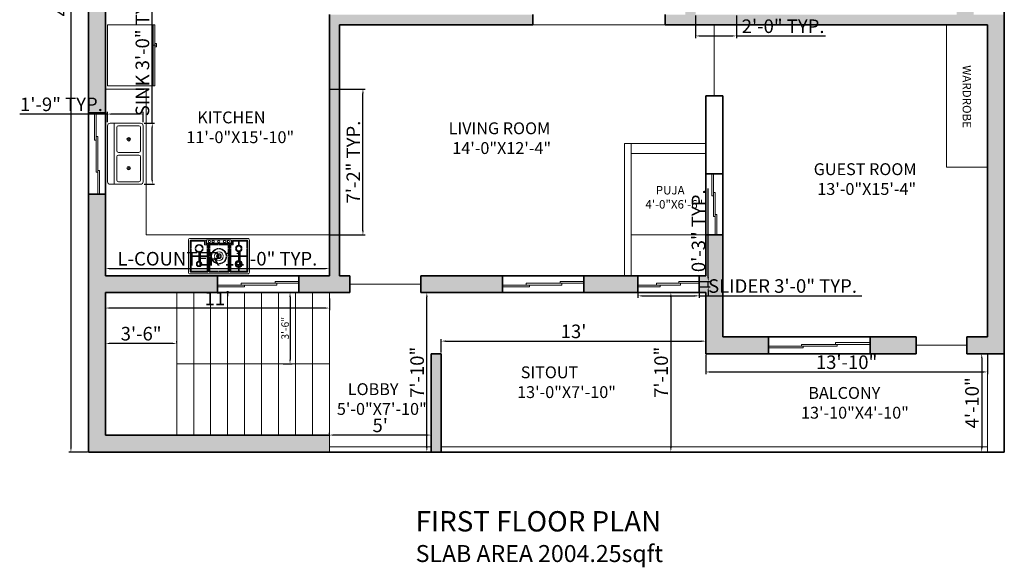
# Model space of a CAD drawing. Units: inches. Extents: x 3491 to 6898, y 1360 to 2019.
# Tile 4 of 9: x 4120 to 4700, y 1360 to 1683. Entities that reach past the tile are written whole.
import ezdxf

# ---------------------------------------------------------------- set-up
doc = ezdxf.new("R2010")
doc.units = ezdxf.units.IN
for name, color, linetype, lineweight in [('A-ANNO-DIMS', 2, 'Continuous', 18), ('A-ANNO-TEXT', 7, 'Continuous', 18), ('A-ANNO-TITL', 7, 'Continuous', 30), ('A-AREA-IDEN', 7, 'Continuous', 18), ('A-DOOR', 4, 'Continuous', 18), ('A-EQPM', 8, 'Continuous', 18), ('A-FLOR-CASE', 8, 'Continuous', 18), ('A-FLOR-FIXT', 8, 'Continuous', 18), ('A-FLOR-RAL', 7, 'Continuous', 18), ('A-FLOR-STRS', 7, 'Continuous', 18), ('A-GLAZ', 5, 'Continuous', 18), ('A-WALL', 7, 'Continuous', 35), ('A-WALL-PATT', 8, 'Continuous', 13)]:
    doc.layers.add(name, color=color, linetype=linetype, lineweight=lineweight)
doc.layers.add('A-WALL-OPEN', color=251, linetype='Continuous', lineweight=13, true_color=0x636466)
doc.styles.get("Standard").update_dxf_attribs({"font": 'arial.ttf'})
doc.dimstyles.new('ISO-25', dxfattribs={"dimtxt": 8, "dimasz": 2.5, "dimexe": 1.25, "dimexo": 0.625, "dimtad": 1, "dimdec": 1, "dimlunit": 3, "dimtxsty": 'Standard', "dimcen": 2.5, "dimclrt": 1, "dimadec": 0, "dimazin": 0, "dimtfac": 1, "dimtdec": 1, "dimtmove": 0, "dimatfit": 3, "dimfxl": 1, "dimarcsym": 0})

# ---------------------------------------------------------------- blocks, each defined once
blk = doc.blocks.new('*D17')
at = {"layer": 'A-ANNO-DIMS', "color": 0, "lineweight": -2, "transparency": 16777216}
for p, q in [((4159.68, 1972.37), (4148.67, 1972.37)), ((4149.92, 1969.87), (4149.92, 1430.87)), ((4159.68, 1428.37), (4148.67, 1428.37))]:
    blk.add_line(p, q, dxfattribs=at)
at = {"layer": 'A-ANNO-DIMS', "color": 0, "transparency": 16777216}
for points in [[(4149.51, 1969.87), (4150.34, 1969.87), (4149.92, 1972.37)], [(4149.51, 1430.87), (4150.34, 1430.87), (4149.92, 1428.37)]]:
    blk.add_solid(points, dxfattribs=at)
at = {"layer": 'Defpoints', "color": 0, "transparency": 16777216}
for p in [(4160.3, 1972.37), (4149.92, 1428.37), (4160.3, 1428.37)]:
    blk.add_point(p, dxfattribs=at)
at = {"layer": 'A-ANNO-DIMS', "color": 0, "transparency": 16777216, "insert": (4145.23, 1700.37), "char_height": 8, "attachment_point": 5, "rotation": 90}
blk.add_mtext('45\'-4"', dxfattribs=at)
blk = doc.blocks.new('*D14')
at = {"layer": 'A-ANNO-DIMS', "color": 0, "lineweight": -2, "transparency": 16777216}
for p, q in [((4170.3, 1493.03), (4170.3, 1493.65)), ((4209.8, 1492.4), (4172.8, 1492.4)), ((4212.3, 1493.03), (4212.3, 1493.65))]:
    blk.add_line(p, q, dxfattribs=at)
at = {"layer": 'A-ANNO-DIMS', "color": 0, "transparency": 16777216}
for points in [[(4172.8, 1492.82), (4172.8, 1491.99), (4170.3, 1492.4)], [(4209.8, 1492.82), (4209.8, 1491.99), (4212.3, 1492.4)]]:
    blk.add_solid(points, dxfattribs=at)
at = {"layer": 'Defpoints', "color": 0, "transparency": 16777216}
for p in [(4170.3, 1492.4), (4170.3, 1492.4), (4212.3, 1492.4)]:
    blk.add_point(p, dxfattribs=at)
at = {"layer": 'A-ANNO-DIMS', "color": 0, "transparency": 16777216, "insert": (4191.3, 1497.12), "char_height": 8, "attachment_point": 5}
blk.add_mtext('3\'-6"', dxfattribs=at)
blk = doc.blocks.new('*D12')
at = {"layer": 'A-ANNO-DIMS', "color": 0, "lineweight": -2, "transparency": 16777216}
for p, q in [((4275.02, 1522.37), (4280.36, 1522.37)), ((4279.11, 1519.87), (4279.11, 1482.87)), ((4275.02, 1480.37), (4280.36, 1480.37))]:
    blk.add_line(p, q, dxfattribs=at)
at = {"layer": 'A-ANNO-DIMS', "color": 0, "transparency": 16777216}
for points in [[(4278.69, 1519.87), (4279.53, 1519.87), (4279.11, 1522.37)], [(4278.69, 1482.87), (4279.53, 1482.87), (4279.11, 1480.37)]]:
    blk.add_solid(points, dxfattribs=at)
at = {"layer": 'Defpoints', "color": 0, "transparency": 16777216}
for p in [(4274.39, 1522.37), (4274.39, 1480.37), (4279.11, 1480.37)]:
    blk.add_point(p, dxfattribs=at)
at = {"layer": 'A-ANNO-DIMS', "color": 0, "transparency": 16777216, "insert": (4276.22, 1501.37), "char_height": 8, "attachment_point": 5, "rotation": 90}
blk.add_mtext('{\\H0.55556x;3\'-6"}', dxfattribs=at)
blk = doc.blocks.new('STOVE')
for p, q in [((11.85, 19.7), (11.55, 19.7)), ((11.55, 16.92), (11.55, 19.7)), ((11.85, 16.92), (11.85, 19.7)), ((-11.85, 13.73), (-11.85, 7.62)), ((-11.85, 13.73), (-11.55, 13.73)), ((-11.55, 13.73), (-11.55, 7.62)), ((11.85, 16.92), (11.55, 16.92)), ((11.85, 13.23), (11.55, 13.23)), ((11.55, 13.23), (11.55, 7.57)), ((11.85, 13.23), (11.85, 7.57)), ((-11.85, 10.75), (-16.4, 10.75)), ((-11.85, 10.25), (-16.4, 10.25)), ((-11.85, 7.62), (-11.55, 7.62)), ((-7, 10.75), (-11.55, 10.75)), ((-7, 10.25), (-11.55, 10.25)), ((7, 10.75), (11.55, 10.75)), ((7, 10.25), (11.55, 10.25)), ((11.85, 7.57), (11.55, 7.57)), ((11.85, 10.75), (16.4, 10.75)), ((11.85, 10.25), (16.4, 10.25)), ((-7, 3.9), (-8.4, 3.9)), ((-7.8, 3.3), (-7.8, 1)), ((-6.4, 3.3), (-7.8, 3.3)), ((7.3, 2.8), (-7.3, 2.8)), ((-7.3, 2.8), (-7.3, 0.8)), ((7.3, 0.8), (-7.3, 0.8)), ((-5.4, 3.9), (-6, 3.9)), ((-5.4, 3.9), (-0.15, 3.9)), ((0.15, 3.9), (5.4, 3.9)), ((6.4, 3.3), (7.8, 3.3)), ((7, 3.9), (8.4, 3.9)), ((7.3, 2.8), (7.3, 0.8)), ((7.8, 3.3), (7.8, 1)), ((8.4, 3.9), (8.4, 1.6)), ((11.85, 4.28), (11.55, 4.28)), ((11.55, 4.28), (11.55, 1.3)), ((11.85, 1.3), (11.55, 1.3)), ((11.85, 4.28), (11.85, 1.3))]:
    blk.add_line(p, q)
for points in [[(-17, 21), (17, 21, -0.414214), (18, 20), (18, 1, -0.414214), (17, 0), (-17, 0, -0.414214), (-18, 1), (-18, 20, -0.414214)], [(6, 3.3), (-6, 3.3), (-6, 19.4, -0.414214), (-5.4, 20), (5.4, 20, -0.414214), (6, 19.4)]]:
    blk.add_lwpolyline(points, format="xyb", close=True)
for points in [[(-7.8, 1), (-16.4, 1, -0.414214), (-17, 1.6), (-17, 19.4, -0.414214), (-16.4, 20), (-7, 20, -0.414214), (-6.4, 19.4), (-6.4, 3.3)], [(6.4, 19.4, -0.414214), (7, 20), (16.4, 20, -0.414214), (17, 19.4), (17, 1.6, -0.414214), (16.4, 1), (7.8, 1)]]:
    blk.add_lwpolyline(points, format="xyb")
for points in [[(-16.4, 15.22), (-16.4, 19.4), (-11.85, 19.4)], [(-11.55, 19.4), (-7, 19.4), (-7, 15.22)], [(-5.4, 15.22), (-5.4, 19.4), (-0.15, 19.4)], [(0.15, 19.4), (5.4, 19.4), (5.4, 15.22)], [(6.4, 3.3), (6.4, 19.4)], [(7, 15.22), (7, 19.4), (11.55, 19.4)], [(11.85, 19.4), (16.4, 19.4), (16.4, 15.22)], [(-16.4, 6.08), (-16.4, 14.92)], [(-7, 14.92), (-7, 6.08)], [(-5.4, 10.65), (-5.4, 14.92)], [(5.4, 14.92), (5.4, 10.65)], [(7, 6.08), (7, 14.92)], [(16.4, 14.92), (16.4, 6.08)], [(-5.4, 6.08), (-5.4, 10.35)], [(5.4, 10.35), (5.4, 6.08)], [(-11.85, 1.6), (-16.4, 1.6), (-16.4, 5.77)], [(-8.4, 3.9), (-8.4, 1.6), (-11.55, 1.6)], [(-7, 5.77), (-7, 3.9)], [(-5.4, 3.9), (-5.4, 5.77)], [(5.4, 5.77), (5.4, 3.9)], [(7, 3.9), (7, 5.77)], [(11.55, 1.6), (8.4, 1.6)], [(16.4, 5.77), (16.4, 1.6), (11.85, 1.6)]]:
    blk.add_lwpolyline(points)
for centre, radius in [((-11.7, 15.07), 1.1), ((0, 10.5), 1.4), ((11.7, 15.07), 1.6), ((11.7, 15.07), 1.1), ((0, 10.5), 0.8), ((11.7, 5.93), 1.4), ((-5.49, 1.8), 0.6), ((-3.3, 1.8), 0.6), ((0, 1.8), 0.6), ((3.39, 1.8), 0.6), ((5.57, 1.8), 0.6)]:
    blk.add_circle(centre, radius)
for centre, radius, start, end in [((-11.7, 15.07), 1.6, 95.37938, 174.62062), ((-11.7, 15.07), 1.6, 185.37938, 264.62062), ((-11.7, 15.07), 1.6, 5.37938, 84.62062), ((-11.7, 15.07), 1.6, 275.37938, 354.62062), ((0, 10.5), 4.6, 91.86867, 178.13133), ((0, 10.5), 4.3, 91.9991, 178.0009), ((0, 10.5), 2.6, 93.30736, 176.69264), ((0, 10.5), 4.6, 1.86867, 88.13133), ((0, 10.5), 4.3, 1.9991, 88.0009), ((0, 10.5), 2.6, 3.30736, 86.69264), ((11.7, 15.07), 2.1, 94.09604, 175.90396), ((11.7, 15.07), 2.1, 184.09604, 265.90396), ((11.7, 15.07), 2.1, 4.09604, 85.90396), ((11.7, 15.07), 2.1, 274.09604, 355.90396), ((-11.7, 5.93), 2.4, 93.58332, 176.41668), ((-11.7, 5.93), 2, 94.30122, 175.69878), ((-11.7, 5.93), 2.4, 3.58332, 86.41668), ((-11.7, 5.93), 2, 4.30122, 85.69878), ((0, 10.5), 4.6, 181.86867, 268.13133), ((0, 10.5), 4.3, 181.9991, 268.0009), ((0, 10.5), 2.6, 183.30736, 266.69264), ((0, 10.5), 4.6, 271.86867, 358.13133), ((0, 10.5), 4.3, 271.9991, 358.0009), ((0, 10.5), 2.6, 273.30736, 356.69264), ((11.7, 5.93), 1.9, 94.52806, 175.47194), ((11.7, 5.93), 1.9, 4.52806, 85.47194), ((-11.7, 5.93), 2.4, 183.58332, 266.41668), ((-11.7, 5.93), 2, 184.30122, 265.69878), ((-11.7, 5.93), 2.4, 273.58332, 356.41668), ((-11.7, 5.93), 2, 274.30122, 355.69878), ((-5.49, 1.8), 0.846, 89.99794, 270), ((-3.3, 1.8), 0.846, 89.99794, 270), ((0, 1.8), 0.846, 89.99794, 270), ((3.39, 1.8), 0.846, 89.99794, 270), ((5.57, 1.8), 0.846, 89.99794, 270), ((11.7, 5.93), 1.9, 184.52806, 265.47194), ((11.7, 5.93), 1.9, 274.52806, 355.47194)]:
    blk.add_arc(centre, radius, start, end)
blk = doc.blocks.new('Sink-double - 36 in top')
for p, q in [((-18, -4), (18, -4)), ((-0.75, -18.5), (-0.75, -6.5)), ((0.75, -6.5), (0.75, -18.5))]:
    blk.add_line(p, q)
for points in [[(-16.5, 0), (16.5, 0)], [(-18, -19.5), (-18, -1.5)], [(-15.5, -5.5), (-1.75, -5.5)], [(1.75, -5.5), (15.5, -5.5)], [(18, -1.5), (18, -19.5)], [(-16.5, -18.5), (-16.5, -6.5)], [(16.5, -6.5), (16.5, -18.5)], [(16.5, -21), (-16.5, -21)], [(-1.75, -19.5), (-15.5, -19.5)], [(15.5, -19.5), (1.75, -19.5)]]:
    blk.add_lwpolyline(points)
for centre, radius in [((-8.5, -12.5), 1), ((8.5, -12.5), 1), ((-8.5, -12.5), 0.5), ((8.5, -12.5), 0.5)]:
    blk.add_circle(centre, radius)
for centre, radius, start, end in [((-16.5, -1.5), 1.5, 90, 180), ((16.5, -1.5), 1.5, 0, 90), ((-15.5, -6.5), 1, 90, 180), ((-1.75, -6.5), 1, 0, 90), ((1.75, -6.5), 1, 90, 180), ((15.5, -6.5), 1, 0, 90), ((-16.5, -19.5), 1.5, 180, 270), ((-15.5, -18.5), 1, 180, 270), ((-1.75, -18.5), 1, 270, 0), ((1.75, -18.5), 1, 180, 270), ((15.5, -18.5), 1, 270, 0), ((16.5, -19.5), 1.5, 270, 0)]:
    blk.add_arc(centre, radius, start, end)
blk = doc.blocks.new('Refrigerator-2 door - 36 in top')
for p, q in [((0, -26.999999), (36, -26.999999)), ((11, -27.999999), (11, -28.999999)), ((11, -28.999999), (13, -28.999999)), ((12, -26.999999), (12, -28.999999)), ((13, -28.999999), (13, -27.999999))]:
    blk.add_line(p, q)
blk.add_lwpolyline([(0, -27.999999), (0, 0), (36, 0), (36, -27.999999)], close=True)
blk = doc.blocks.new('*D18')
at = {"layer": 'A-ANNO-DIMS', "color": 0, "lineweight": -2, "transparency": 16777216}
for p, q in [((4170.3, 1521.74), (4170.3, 1512.03)), ((4302.3, 1518.98), (4302.3, 1512.03)), ((4299.8, 1513.28), (4172.8, 1513.28))]:
    blk.add_line(p, q, dxfattribs=at)
at = {"layer": 'A-ANNO-DIMS', "color": 0, "transparency": 16777216}
for points in [[(4172.8, 1513.7), (4172.8, 1512.87), (4170.3, 1513.28)], [(4299.8, 1513.7), (4299.8, 1512.87), (4302.3, 1513.28)]]:
    blk.add_solid(points, dxfattribs=at)
at = {"layer": 'Defpoints', "color": 0, "transparency": 16777216}
for p in [(4170.3, 1522.37), (4302.3, 1519.61), (4170.3, 1513.28)]:
    blk.add_point(p, dxfattribs=at)
at = {"layer": 'A-ANNO-DIMS', "color": 0, "transparency": 16777216, "insert": (4236.3, 1517.92), "char_height": 8, "attachment_point": 5}
blk.add_mtext("11'", dxfattribs=at)
blk = doc.blocks.new('*D19')
at = {"layer": 'A-ANNO-DIMS', "color": 0, "lineweight": -2, "transparency": 16777216}
for p, q in [((4524.3, 1485.74), (4524.3, 1474.33)), ((4690.3, 1485.74), (4690.3, 1474.33)), ((4526.8, 1475.58), (4687.8, 1475.58))]:
    blk.add_line(p, q, dxfattribs=at)
at = {"layer": 'A-ANNO-DIMS', "color": 0, "transparency": 16777216}
for points in [[(4526.8, 1476), (4526.8, 1475.16), (4524.3, 1475.58)], [(4687.8, 1476), (4687.8, 1475.16), (4690.3, 1475.58)]]:
    blk.add_solid(points, dxfattribs=at)
at = {"layer": 'Defpoints', "color": 0, "transparency": 16777216}
for p in [(4524.3, 1486.37), (4690.3, 1486.37), (4690.3, 1475.58)]:
    blk.add_point(p, dxfattribs=at)
at = {"layer": 'A-ANNO-DIMS', "color": 0, "transparency": 16777216, "insert": (4607.3, 1480.29), "char_height": 8, "attachment_point": 5}
blk.add_mtext('13\'-10"', dxfattribs=at)
blk = doc.blocks.new('*D20')
at = {"layer": 'A-ANNO-DIMS', "color": 0, "lineweight": -2, "transparency": 16777216}
for p, q in [((4689.68, 1486.37), (4685.75, 1486.37)), ((4687, 1483.87), (4687, 1430.87)), ((4689.68, 1428.37), (4685.75, 1428.37))]:
    blk.add_line(p, q, dxfattribs=at)
at = {"layer": 'A-ANNO-DIMS', "color": 0, "transparency": 16777216}
for points in [[(4686.59, 1483.87), (4687.42, 1483.87), (4687, 1486.37)], [(4686.59, 1430.87), (4687.42, 1430.87), (4687, 1428.37)]]:
    blk.add_solid(points, dxfattribs=at)
at = {"layer": 'Defpoints', "color": 0, "transparency": 16777216}
for p in [(4690.3, 1486.37), (4687, 1428.37), (4690.3, 1428.37)]:
    blk.add_point(p, dxfattribs=at)
at = {"layer": 'A-ANNO-DIMS', "color": 0, "transparency": 16777216, "insert": (4682.29, 1457.37), "char_height": 8, "attachment_point": 5, "rotation": 90}
blk.add_mtext('4\'-10"', dxfattribs=at)
blk = doc.blocks.new('*D21')
at = {"layer": 'A-ANNO-DIMS', "color": 0, "lineweight": -2, "transparency": 16777216}
for p, q in [((4368.3, 1486.99), (4368.3, 1495.02)), ((4370.8, 1493.77), (4521.8, 1493.77)), ((4524.3, 1486.99), (4524.3, 1495.02))]:
    blk.add_line(p, q, dxfattribs=at)
at = {"layer": 'A-ANNO-DIMS', "color": 0, "transparency": 16777216}
for points in [[(4370.8, 1494.19), (4370.8, 1493.35), (4368.3, 1493.77)], [(4521.8, 1494.19), (4521.8, 1493.35), (4524.3, 1493.77)]]:
    blk.add_solid(points, dxfattribs=at)
at = {"layer": 'Defpoints', "color": 0, "transparency": 16777216}
for p in [(4524.3, 1493.77), (4368.3, 1486.37), (4524.3, 1486.37)]:
    blk.add_point(p, dxfattribs=at)
at = {"layer": 'A-ANNO-DIMS', "color": 0, "transparency": 16777216, "insert": (4446.3, 1498.48), "char_height": 8, "attachment_point": 5}
blk.add_mtext("13'", dxfattribs=at)
blk = doc.blocks.new('*D22')
at = {"layer": 'A-ANNO-DIMS', "color": 0, "lineweight": -2, "transparency": 16777216}
for p, q in [((4504.3, 1522.37), (4504.93, 1522.37)), ((4503.68, 1519.87), (4503.68, 1430.87)), ((4504.3, 1428.37), (4504.93, 1428.37))]:
    blk.add_line(p, q, dxfattribs=at)
at = {"layer": 'A-ANNO-DIMS', "color": 0, "transparency": 16777216}
for points in [[(4503.26, 1519.87), (4504.09, 1519.87), (4503.68, 1522.37)], [(4503.26, 1430.87), (4504.09, 1430.87), (4503.68, 1428.37)]]:
    blk.add_solid(points, dxfattribs=at)
at = {"layer": 'Defpoints', "color": 0, "transparency": 16777216}
for p in [(4503.68, 1522.37), (4503.68, 1428.37), (4503.68, 1428.37)]:
    blk.add_point(p, dxfattribs=at)
at = {"layer": 'A-ANNO-DIMS', "color": 0, "transparency": 16777216, "insert": (4498.97, 1475.37), "char_height": 8, "attachment_point": 5, "rotation": 90}
blk.add_mtext('7\'-10"', dxfattribs=at)
blk = doc.blocks.new('*D23')
at = {"layer": 'A-ANNO-DIMS', "color": 0, "lineweight": -2, "transparency": 16777216}
for p, q in [((4356.93, 1522.37), (4361.04, 1522.37)), ((4359.79, 1430.87), (4359.79, 1519.87)), ((4353.25, 1428.37), (4361.04, 1428.37))]:
    blk.add_line(p, q, dxfattribs=at)
at = {"layer": 'A-ANNO-DIMS', "color": 0, "transparency": 16777216}
for points in [[(4359.38, 1519.87), (4360.21, 1519.87), (4359.79, 1522.37)], [(4359.38, 1430.87), (4360.21, 1430.87), (4359.79, 1428.37)]]:
    blk.add_solid(points, dxfattribs=at)
at = {"layer": 'Defpoints', "color": 0, "transparency": 16777216}
for p in [(4356.3, 1522.37), (4359.79, 1522.37), (4352.62, 1428.37)]:
    blk.add_point(p, dxfattribs=at)
at = {"layer": 'A-ANNO-DIMS', "color": 0, "transparency": 16777216, "insert": (4355.08, 1475.37), "char_height": 8, "attachment_point": 5, "rotation": 90}
blk.add_mtext('7\'-10"', dxfattribs=at)
blk = doc.blocks.new('*D24')
at = {"layer": 'A-ANNO-DIMS', "color": 0, "lineweight": -2, "transparency": 16777216}
for p, q in [((4302.3, 1438.99), (4302.3, 1439.62)), ((4359.8, 1438.37), (4304.8, 1438.37)), ((4362.3, 1438.46), (4362.3, 1439.62))]:
    blk.add_line(p, q, dxfattribs=at)
at = {"layer": 'A-ANNO-DIMS', "color": 0, "transparency": 16777216}
for points in [[(4304.8, 1438.78), (4304.8, 1437.95), (4302.3, 1438.37)], [(4359.8, 1438.78), (4359.8, 1437.95), (4362.3, 1438.37)]]:
    blk.add_solid(points, dxfattribs=at)
at = {"layer": 'Defpoints', "color": 0, "transparency": 16777216}
for p in [(4302.3, 1438.37), (4302.3, 1438.37), (4362.3, 1437.84)]:
    blk.add_point(p, dxfattribs=at)
at = {"layer": 'A-ANNO-DIMS', "color": 0, "transparency": 16777216, "insert": (4332.3, 1443.06), "char_height": 8, "attachment_point": 5}
blk.add_mtext("5'", dxfattribs=at)
blk = doc.blocks.new('WIN-SLIDER-48IN')
for p, q in [((35, 1), (0, 1)), ((48, 2), (14, 2)), ((14, 2), (14, 1)), ((16, 1), (16, 0)), ((34, 3), (34, 2)), ((48, 3), (34, 3)), ((35, 2), (35, 1)), ((16, 0), (0, 0))]:
    blk.add_line(p, q)
blk = doc.blocks.new('WIN-SLIDER-36IN')
for p, q in [((25, 1), (0, 1)), ((13, 0), (0, 0)), ((36, 2), (11, 2)), ((11, 2), (11, 1)), ((13, 1), (13, 0)), ((24, 3), (24, 2)), ((36, 3), (24, 3)), ((25, 2), (25, 1))]:
    blk.add_line(p, q)
blk = doc.blocks.new('WIN-SLIDER-60IN')
for p, q in [((0, 39.5), (0, 60)), ((1, 19.5), (1, 60)), ((1, 39.5), (0, 39.5)), ((2, 40.5), (1, 40.5)), ((2, 0), (2, 40.5)), ((2, 19.5), (1, 19.5)), ((3, 20.5), (2, 20.5)), ((3, 0), (3, 20.5))]:
    blk.add_line(p, q)
blk = doc.blocks.new('STAIR-RETURN-FLIGHT')
for p, q in [((0, 84), (0, 0)), ((10, 84), (10, 0)), ((20, 84), (20, 0)), ((30, 84), (30, 0)), ((40, 84), (40, 0)), ((50, 84), (50, 0)), ((60, 84), (60, 0)), ((70, 84), (70, 0)), ((80, 84), (80, 0)), ((0, 42), (90, 42))]:
    blk.add_line(p, q)
blk = doc.blocks.new('COUNTER-KITCHEN-L')
for p, q in [((24, 86.04), (0, 86.04)), ((24, 86.04), (24, 0)), ((132, 0), (24, 0))]:
    blk.add_line(p, q)
blk = doc.blocks.new('PUJA-ALCOVE-48X78')
for p, q in [((0, 78), (0, 0)), ((48, 78), (0, 78)), ((4, 78), (4, 0)), ((48, 72), (4, 72)), ((48, 24), (4, 24))]:
    blk.add_line(p, q)
blk = doc.blocks.new('WARDROBE-84X24')
for q in [(0, 84), (24, 0)]:
    blk.add_line((24, 84), q)
blk = doc.blocks.new('*D116')
at = {"layer": 'A-ANNO-DIMS', "color": 0, "lineweight": -2, "transparency": 16777216}
for p, q in [((4484.3, 1525.24), (4484.3, 1519.22)), ((4520.3, 1525.24), (4520.3, 1519.22)), ((4486.8, 1520.47), (4517.8, 1520.47)), ((4520.3, 1520.47), (4616.26, 1520.47))]:
    blk.add_line(p, q, dxfattribs=at)
at = {"layer": 'A-ANNO-DIMS', "color": 0, "transparency": 16777216}
for points in [[(4486.8, 1520.88), (4486.8, 1520.05), (4484.3, 1520.47)], [(4517.8, 1520.88), (4517.8, 1520.05), (4520.3, 1520.47)]]:
    blk.add_solid(points, dxfattribs=at)
at = {"layer": 'Defpoints', "color": 0, "transparency": 16777216}
for p in [(4484.3, 1525.87), (4520.3, 1525.87), (4520.3, 1520.47)]:
    blk.add_point(p, dxfattribs=at)
at = {"layer": 'A-ANNO-DIMS', "color": 1, "transparency": 16777216, "insert": (4569.53, 1525.23), "char_height": 8, "attachment_point": 5}
blk.add_mtext('SLIDER 3\'-0" TYP.', dxfattribs=at)
blk = doc.blocks.new('*D117')
at = {"layer": 'A-ANNO-DIMS', "color": 0, "lineweight": -2, "transparency": 16777216}
for p, q in [((4525.7, 1531.37), (4525.7, 1583.88)), ((4520.93, 1528.87), (4526.95, 1528.87)), ((4525.7, 1525.87), (4525.7, 1528.87)), ((4520.93, 1525.87), (4526.95, 1525.87)), ((4525.7, 1523.37), (4525.7, 1520.87))]:
    blk.add_line(p, q, dxfattribs=at)
at = {"layer": 'A-ANNO-DIMS', "color": 0, "transparency": 16777216}
for points in [[(4525.29, 1531.37), (4526.12, 1531.37), (4525.7, 1528.87)], [(4525.29, 1523.37), (4526.12, 1523.37), (4525.7, 1525.87)]]:
    blk.add_solid(points, dxfattribs=at)
at = {"layer": 'Defpoints', "color": 0, "transparency": 16777216}
for p in [(4520.3, 1528.87), (4525.7, 1528.87), (4520.3, 1525.87)]:
    blk.add_point(p, dxfattribs=at)
at = {"layer": 'A-ANNO-DIMS', "color": 1, "transparency": 16777216, "insert": (4520.99, 1558.87), "char_height": 8, "attachment_point": 5, "rotation": 90}
blk.add_mtext('0\'-3" TYP.', dxfattribs=at)
blk = doc.blocks.new('*D123')
at = {"layer": 'A-ANNO-DIMS', "color": 0, "lineweight": -2, "transparency": 16777216}
for p, q in [((4518.3, 1685.74), (4518.3, 1672.52)), ((4542.3, 1685.74), (4542.3, 1672.52)), ((4520.8, 1673.77), (4539.8, 1673.77)), ((4542.3, 1673.77), (4594.96, 1673.77))]:
    blk.add_line(p, q, dxfattribs=at)
at = {"layer": 'A-ANNO-DIMS', "color": 0, "transparency": 16777216}
for points in [[(4520.8, 1674.18), (4520.8, 1673.35), (4518.3, 1673.77)], [(4539.8, 1674.18), (4539.8, 1673.35), (4542.3, 1673.77)]]:
    blk.add_solid(points, dxfattribs=at)
at = {"layer": 'Defpoints', "color": 0, "transparency": 16777216}
for p in [(4518.3, 1686.37), (4542.3, 1686.37), (4542.3, 1673.77)]:
    blk.add_point(p, dxfattribs=at)
at = {"layer": 'A-ANNO-DIMS', "color": 1, "transparency": 16777216, "insert": (4569.88, 1678.48), "char_height": 8, "attachment_point": 5}
blk.add_mtext('2\'-0" TYP.', dxfattribs=at)
blk = doc.blocks.new('*D126')
at = {"layer": 'A-ANNO-DIMS', "color": 0, "lineweight": -2, "transparency": 16777216}
for p, q in [((4197.86, 1622.3), (4197.86, 1703.97)), ((4193.08, 1622.3), (4199.11, 1622.3)), ((4197.86, 1588.8), (4197.86, 1619.8)), ((4193.08, 1586.3), (4199.11, 1586.3))]:
    blk.add_line(p, q, dxfattribs=at)
at = {"layer": 'A-ANNO-DIMS', "color": 0, "transparency": 16777216}
for points in [[(4197.44, 1619.8), (4198.27, 1619.8), (4197.86, 1622.3)], [(4197.44, 1588.8), (4198.27, 1588.8), (4197.86, 1586.3)]]:
    blk.add_solid(points, dxfattribs=at)
at = {"layer": 'Defpoints', "color": 0, "transparency": 16777216}
for p in [(4192.46, 1622.3), (4197.86, 1622.3), (4192.46, 1586.3)]:
    blk.add_point(p, dxfattribs=at)
at = {"layer": 'A-ANNO-DIMS', "color": 1, "transparency": 16777216, "insert": (4193.09, 1664.39), "char_height": 8, "attachment_point": 5, "rotation": 90}
blk.add_mtext('SINK 3\'-0" TYP.', dxfattribs=at)
blk = doc.blocks.new('*D127')
at = {"layer": 'A-ANNO-DIMS', "color": 0, "lineweight": -2, "transparency": 16777216}
for p, q in [((4171.46, 1627.7), (4119.7, 1627.7)), ((4171.46, 1622.93), (4171.46, 1628.95)), ((4189.96, 1627.7), (4173.96, 1627.7)), ((4192.46, 1622.93), (4192.46, 1628.95))]:
    blk.add_line(p, q, dxfattribs=at)
at = {"layer": 'A-ANNO-DIMS', "color": 0, "transparency": 16777216}
for points in [[(4173.96, 1628.12), (4173.96, 1627.29), (4171.46, 1627.7)], [(4189.96, 1628.12), (4189.96, 1627.29), (4192.46, 1627.7)]]:
    blk.add_solid(points, dxfattribs=at)
at = {"layer": 'Defpoints', "color": 0, "transparency": 16777216}
for p in [(4171.46, 1627.7), (4171.46, 1622.3), (4192.46, 1622.3)]:
    blk.add_point(p, dxfattribs=at)
at = {"layer": 'A-ANNO-DIMS', "color": 1, "transparency": 16777216, "insert": (4144.33, 1632.41), "char_height": 8, "attachment_point": 5}
blk.add_mtext('1\'-9" TYP.', dxfattribs=at)
blk = doc.blocks.new('*D132')
at = {"layer": 'A-ANNO-DIMS', "color": 0, "lineweight": -2, "transparency": 16777216}
for p, q in [((4170.3, 1555.74), (4170.3, 1535.32)), ((4302.3, 1555.74), (4302.3, 1535.32)), ((4172.8, 1536.57), (4299.8, 1536.57))]:
    blk.add_line(p, q, dxfattribs=at)
at = {"layer": 'A-ANNO-DIMS', "color": 0, "transparency": 16777216}
for points in [[(4172.8, 1536.98), (4172.8, 1536.15), (4170.3, 1536.57)], [(4299.8, 1536.98), (4299.8, 1536.15), (4302.3, 1536.57)]]:
    blk.add_solid(points, dxfattribs=at)
at = {"layer": 'Defpoints', "color": 0, "transparency": 16777216}
for p in [(4170.3, 1556.37), (4302.3, 1556.37), (4302.3, 1536.57)]:
    blk.add_point(p, dxfattribs=at)
at = {"layer": 'A-ANNO-DIMS', "color": 1, "transparency": 16777216, "insert": (4236.3, 1541.33), "char_height": 8, "attachment_point": 5}
blk.add_mtext('L-COUNTER 11\'-0" TYP.', dxfattribs=at)
blk = doc.blocks.new('*D133')
at = {"layer": 'A-ANNO-DIMS', "color": 0, "lineweight": -2, "transparency": 16777216}
for p, q in [((4302.93, 1642.41), (4323.35, 1642.41)), ((4322.1, 1558.87), (4322.1, 1639.91)), ((4302.93, 1556.37), (4323.35, 1556.37))]:
    blk.add_line(p, q, dxfattribs=at)
at = {"layer": 'A-ANNO-DIMS', "color": 0, "transparency": 16777216}
for points in [[(4321.69, 1639.91), (4322.52, 1639.91), (4322.1, 1642.41)], [(4321.69, 1558.87), (4322.52, 1558.87), (4322.1, 1556.37)]]:
    blk.add_solid(points, dxfattribs=at)
at = {"layer": 'Defpoints', "color": 0, "transparency": 16777216}
for p in [(4302.3, 1642.41), (4322.1, 1642.41), (4302.3, 1556.37)]:
    blk.add_point(p, dxfattribs=at)
at = {"layer": 'A-ANNO-DIMS', "color": 1, "transparency": 16777216, "insert": (4317.46, 1599.39), "char_height": 8, "attachment_point": 5, "rotation": 90}
blk.add_mtext('7\'-2" TYP.', dxfattribs=at)

msp = doc.modelspace()

# ---------------------------------------------------------------- hatches: boundary and pattern name
at = {"layer": 'A-WALL-PATT'}
h = msp.add_hatch(color=256, dxfattribs=at)
h.dxf.hatch_style = 1
h.paths.add_polyline_path([(4484.3, 1532.37), (4476.3, 1532.37), (4452.32, 1532.37), (4452.32, 1522.37), (4484.3, 1522.37)])
h.paths.add_polyline_path([(4534.3, 1556.37), (4524.3, 1556.37), (4524.3, 1532.37), (4520.3, 1532.37), (4520.3, 1522.37), (4524.3, 1522.37), (4524.3, 1486.37), (4561.28, 1486.37), (4561.28, 1496.37), (4534.3, 1496.37)], flags=17)
h.paths.add_polyline_path([(4404.32, 1532.37), (4356.3, 1532.37), (4356.3, 1522.37), (4404.32, 1522.37)], flags=17)
h.paths.add_polyline_path([(4648.3, 1496.37), (4621.28, 1496.37), (4621.28, 1486.37), (4648.3, 1486.37)], flags=17)
h.paths.add_polyline_path([(4700.3, 1686.37), (4682.3, 1686.37), (4682.3, 1719.37), (4672.3, 1719.37), (4672.3, 1686.37), (4518.3, 1686.37), (4518.3, 1776.37), (4512.3, 1776.37), (4512.3, 1686.37), (4500.3, 1686.37), (4500.3, 1680.37), (4690.3, 1680.37), (4690.3, 1496.37), (4678.3, 1496.37), (4678.3, 1486.37), (4700.3, 1486.37)])
h.paths.add_polyline_path([(4422.3, 1686.37), (4302.3, 1686.37), (4302.3, 1532.37), (4284.33, 1532.37), (4284.33, 1522.37), (4314.3, 1522.37), (4314.3, 1532.37), (4308.3, 1532.37), (4308.3, 1680.37), (4422.3, 1680.37)])
h.paths.add_polyline_path([(4170.3, 1722.37), (4248.3, 1722.37), (4248.3, 1782.37), (4242.3, 1782.37), (4242.3, 1728.37), (4170.3, 1728.37), (4170.3, 1770.37), (4160.3, 1770.37), (4160.3, 1628.4), (4170.3, 1628.4)])
h.paths.add_polyline_path([(4170.3, 1580.4), (4160.3, 1580.4), (4160.3, 1428.37), (4302.3, 1428.37), (4302.3, 1438.37), (4170.3, 1438.37), (4170.3, 1522.37), (4236.33, 1522.37), (4236.33, 1532.37), (4170.3, 1532.37)])
h.paths.add_polyline_path([(4368.3, 1486.37), (4362.3, 1486.37), (4362.3, 1428.37), (4368.3, 1428.37)])
h.paths.add_polyline_path([(4682.3, 1857.37), (4672.3, 1857.37), (4672.3, 1818.37), (4512.3, 1818.37), (4512.3, 1812.37), (4672.3, 1812.37), (4672.3, 1779.37), (4682.3, 1779.37)])
h.paths.add_polyline_path([(4476.3, 1872.37), (4470.3, 1872.37), (4470.3, 1818.37), (4410.3, 1818.37), (4410.3, 1902.37), (4428.3, 1902.37), (4428.3, 1908.37), (4386.3, 1908.37), (4386.3, 1902.37), (4404.3, 1902.37), (4404.3, 1818.37), (4344.3, 1818.37), (4344.3, 1872.37), (4338.3, 1872.37), (4338.3, 1812.37), (4476.3, 1812.37)])
h.paths.add_polyline_path([(4170.3, 1857.37), (4160.3, 1857.37), (4160.3, 1794.37), (4170.3, 1794.37), (4170.3, 1812.37), (4302.3, 1812.37), (4302.3, 1818.37), (4170.3, 1818.37)])
h.paths.add_polyline_path([(4170.3, 1962.37), (4338.3, 1962.37), (4338.3, 1938.37), (4344.3, 1938.37), (4344.3, 1962.37), (4470.3, 1962.37), (4470.3, 1938.37), (4476.3, 1938.37), (4476.3, 1962.37), (4672.3, 1962.37), (4672.3, 1923.37), (4682.3, 1923.37), (4682.3, 1972.37), (4160.3, 1972.37), (4160.3, 1923.37), (4170.3, 1923.37)])
h.paths.add_polyline_path([(4476.3, 1908.37), (4452.3, 1908.37), (4452.3, 1902.37), (4476.3, 1902.37)], flags=17)
h.paths.add_polyline_path([(4362.3, 1908.37), (4338.3, 1908.37), (4338.3, 1902.37), (4362.3, 1902.37)], flags=17)

# ---------------------------------------------------------------- linework, layer by layer
at = {"layer": 'A-DOOR'}
for p, q in [((4529.3, 1638.37), (4529.3, 1680.37)), ((4356.3, 1527.37), (4314.3, 1527.37)), ((4678.3, 1491.37), (4648.3, 1491.37))]:
    msp.add_line(p, q, dxfattribs=at)
at = {"layer": 'A-FLOR-RAL'}
for p, q in [((4690.3, 1486.37), (4690.3, 1428.37)), ((4302.3, 1431.37), (4362.3, 1431.37)), ((4368.3, 1431.37), (4690.3, 1431.37))]:
    msp.add_line(p, q, dxfattribs=at)
at = {"layer": 'A-FLOR-STRS'}
msp.add_line((4302.3, 1522.37), (4302.3, 1428.37), dxfattribs=at)
at = {"layer": 'A-WALL'}
for p, q in [((4160.3, 1972.37), (4160.3, 1428.37)), ((4700.3, 1428.37), (4700.3, 1972.37)), ((4170.3, 1722.37), (4170.3, 1532.37)), ((4302.3, 1686.37), (4302.3, 1532.37)), ((4422.3, 1686.37), (4422.3, 1680.37)), ((4500.3, 1686.37), (4500.3, 1680.37)), ((4422.3, 1680.37), (4308.3, 1680.37)), ((4308.3, 1680.37), (4308.3, 1532.37)), ((4690.3, 1680.37), (4500.3, 1680.37)), ((4690.3, 1496.37), (4690.3, 1680.37)), ((4534.3, 1638.37), (4524.3, 1638.37)), ((4524.3, 1638.37), (4524.3, 1532.37)), ((4534.3, 1638.37), (4534.3, 1496.37)), ((4170.3, 1628.4), (4160.3, 1628.4)), ((4534.3, 1592.37), (4524.3, 1592.37)), ((4170.3, 1580.4), (4160.3, 1580.4)), ((4534.3, 1556.37), (4524.3, 1556.37)), ((4302.3, 1532.37), (4170.3, 1532.37)), ((4236.33, 1532.37), (4236.33, 1522.37)), ((4284.33, 1532.37), (4284.33, 1522.37)), ((4314.3, 1532.37), (4308.3, 1532.37)), ((4314.3, 1532.37), (4314.3, 1522.37)), ((4476.3, 1532.37), (4356.3, 1532.37)), ((4356.3, 1532.37), (4356.3, 1522.37)), ((4404.32, 1532.37), (4404.32, 1522.37)), ((4452.32, 1532.37), (4452.32, 1522.37)), ((4524.3, 1532.37), (4476.3, 1532.37)), ((4484.3, 1532.37), (4484.3, 1522.37)), ((4520.3, 1532.37), (4520.3, 1522.37)), ((4170.3, 1522.37), (4170.3, 1438.37)), ((4314.3, 1522.37), (4170.3, 1522.37)), ((4524.3, 1522.37), (4356.3, 1522.37)), ((4524.3, 1522.37), (4524.3, 1486.37)), ((4648.3, 1496.37), (4534.3, 1496.37)), ((4561.28, 1486.37), (4561.28, 1496.37)), ((4621.28, 1486.37), (4621.28, 1496.37)), ((4648.3, 1486.37), (4648.3, 1496.37)), ((4690.3, 1496.37), (4678.3, 1496.37)), ((4678.3, 1486.37), (4678.3, 1496.37)), ((4362.3, 1486.37), (4362.3, 1428.37)), ((4368.3, 1486.37), (4362.3, 1486.37)), ((4368.3, 1486.37), (4368.3, 1428.37)), ((4648.3, 1486.37), (4524.3, 1486.37)), ((4700.3, 1486.37), (4678.3, 1486.37)), ((4170.3, 1438.37), (4302.3, 1438.37)), ((4160.3, 1428.37), (4700.3, 1428.37))]:
    msp.add_line(p, q, dxfattribs=at)
at = {"layer": 'A-WALL-OPEN'}
msp.add_line((4422.3, 1680.37), (4500.3, 1680.37), dxfattribs=at)

# ---------------------------------------------------------------- block references
at = {"layer": 'A-EQPM', "xscale": -1}
for name, p, rotation in [('Refrigerator-2 door - 36 in top', (4171.45, 1680.37), 90), ('STOVE', (4237.17, 1554.37), 180)]:
    msp.add_blockref(name, p, dxfattribs=dict(at, rotation=rotation))
at = {"layer": 'A-FLOR-CASE', "rotation": 180}
msp.add_blockref('WARDROBE-84X24', (4690.3, 1680.37), dxfattribs=at)
at = {"layer": 'A-FLOR-CASE'}
for name, p in [('COUNTER-KITCHEN-L', (4170.3, 1556.37)), ('PUJA-ALCOVE-48X78', (4476.3, 1532.37))]:
    msp.add_blockref(name, p, dxfattribs=at)
at = {"layer": 'A-FLOR-FIXT', "rotation": 90}
msp.add_blockref('Sink-double - 36 in top', (4171.46, 1604.3), dxfattribs=at)
at = {"layer": 'A-FLOR-STRS'}
msp.add_blockref('STAIR-RETURN-FLIGHT', (4212.3, 1438.37), dxfattribs=at)
at = {"layer": 'A-GLAZ', "rotation": 270}
for name, p in [('WIN-SLIDER-48IN', (4163.8, 1628.4)), ('WIN-SLIDER-36IN', (4527.8, 1592.37)), ('WIN-SLIDER-60IN', (4561.28, 1492.87))]:
    msp.add_blockref(name, p, dxfattribs=at)
at = {"layer": 'A-GLAZ'}
for name, p in [('WIN-SLIDER-48IN', (4236.33, 1525.87)), ('WIN-SLIDER-48IN', (4404.32, 1525.87)), ('WIN-SLIDER-36IN', (4484.3, 1525.87))]:
    msp.add_blockref(name, p, dxfattribs=at)

# ---------------------------------------------------------------- texts
at = {"layer": 'A-ANNO-TEXT', "insert": (4680.75, 1656.53), "char_height": 5, "attachment_point": 1, "rotation": 270}
msp.add_mtext_dynamic_manual_height_columns('WARDROBE', width=86.9528, gutter_width=12.5, heights=[0], dxfattribs=at)
at = {"layer": 'A-ANNO-TITL', "insert": (4353.19, 1393.48), "char_height": 12, "attachment_point": 1}
msp.add_mtext_dynamic_manual_height_columns('FIRST FLOOR PLAN\\P{\\H0.83333x;SLAB AREA 2004.25sqft}', width=285.9409, gutter_width=12.5, heights=[0], dxfattribs=at)
at = {"layer": 'A-AREA-IDEN', "attachment_point": 1}
for s, width, insert, char_height in [('   KITCHEN\\P11\'-0"X15\'-10"', 86.9528, (4217.98, 1629.22), 7), ('LIVING ROOM\\P 14\'-0"X12\'-4"', 121.6144, (4372.66, 1622.81), 7), ('GUEST ROOM\\P 13\'-0"X15\'-4"', 121.6144, (4587.91, 1598.68), 7), ('    PUJA\\P4\'-0"X6\'-6"', 33.0959, (4488.65, 1585.28), 5), (' SITOUT\\P13\'-0"X7\'-10"', 121.6144, (4413.02, 1478.87), 7), ('   LOBBY\\P5\'-0"X7\'-10"', 121.6144, (4306.75, 1468.93), 7), ('  BALCONY\\P13\'-10"X4\'-10"', 121.6144, (4580.45, 1466.71), 7)]:
    msp.add_mtext_dynamic_manual_height_columns(s, width=width, gutter_width=12.5, heights=[0], dxfattribs=dict(at, insert=insert, char_height=char_height))

# ---------------------------------------------------------------- dimensions: what is measured, and where the dimension line sits
at = {"layer": 'A-ANNO-DIMS'}
for base, p1, p2, picture, middle in [((4149.92, 1428.37), (4160.3, 1972.37), (4160.3, 1428.37), '*D17', (4145.23, 1700.37)), ((4359.79, 1522.37), (4352.62, 1428.37), (4356.3, 1522.37), '*D23', (4355.08, 1475.37)), ((4503.68, 1428.37), (4503.68, 1522.37), (4503.68, 1428.37), '*D22', (4498.97, 1475.37)), ((4687, 1428.37), (4690.3, 1486.37), (4690.3, 1428.37), '*D20', (4682.29, 1457.37))]:
    dim = msp.add_linear_dim(base=base, p1=p1, p2=p2, angle=90, dimstyle='ISO-25', override={"dimclrd": 0, "dimclre": 0, "dimclrt": 0}, dxfattribs=at)
    dim.commit()
    dim.dimension.update_dxf_attribs({"geometry": picture, "text_midpoint": middle})
for base, p1, p2, angle, text, override, picture, middle in [((4197.86, 1622.3), (4192.46, 1586.3), (4192.46, 1622.3), 90, 'SINK <> TYP.', {"dimdec": 1, "dimlfac": 1, "dimrnd": 0, "dimzin": 1, "dimdsep": 46, "dimlunit": 4, "dimfrac": 2}, '*D126', (4193.09, 1664.39)), ((4171.46, 1627.7), (4192.46, 1622.3), (4171.46, 1622.3), 180, '<> TYP.', {"dimdec": 1, "dimlfac": 1, "dimrnd": 0, "dimzin": 1, "dimdsep": 46, "dimlunit": 4, "dimfrac": 2}, '*D127', (4144.33, 1632.41)), ((4322.1, 1642.41), (4302.3, 1556.37), (4302.3, 1642.41), 90, '<> TYP.', {"dimdec": 1, "dimlfac": 1, "dimrnd": 0, "dimzin": 1, "dimdsep": 46, "dimlunit": 4, "dimfrac": 2}, '*D133', (4317.46, 1599.39)), ((4525.7, 1528.87), (4520.3, 1525.87), (4520.3, 1528.87), 90, '<> TYP.', {"dimdec": 1, "dimlfac": 1, "dimrnd": 0, "dimzin": 1, "dimdsep": 46, "dimlunit": 4, "dimfrac": 2}, '*D117', (4520.99, 1558.87)), ((4279.11, 1480.37), (4274.39, 1522.37), (4274.39, 1480.37), 90, '{\\H0.55556x;<>}', {"dimclrd": 0, "dimclre": 0, "dimclrt": 0}, '*D12', (4276.22, 1501.37))]:
    dim = msp.add_linear_dim(base=base, p1=p1, p2=p2, angle=angle, text=text, dimstyle='ISO-25', override=override, dxfattribs=at)
    dim.commit()
    dim.dimension.update_dxf_attribs({"geometry": picture, "text_midpoint": middle})
for base, p1, p2, text, picture, middle in [((4542.3, 1673.77), (4518.3, 1686.37), (4542.3, 1686.37), '<> TYP.', '*D123', (4569.88, 1678.48)), ((4302.3, 1536.57), (4170.3, 1556.37), (4302.3, 1556.37), 'L-COUNTER <> TYP.', '*D132', (4236.3, 1541.33)), ((4520.3, 1520.47), (4484.3, 1525.87), (4520.3, 1525.87), 'SLIDER <> TYP.', '*D116', (4569.53, 1525.23))]:
    dim = msp.add_linear_dim(base=base, p1=p1, p2=p2, text=text, dimstyle='ISO-25', override={"dimdec": 1, "dimlfac": 1, "dimrnd": 0, "dimzin": 1, "dimdsep": 46, "dimlunit": 4, "dimfrac": 2}, dxfattribs=at)
    dim.commit()
    dim.dimension.update_dxf_attribs({"geometry": picture, "text_midpoint": middle})
for base, p1, p2, picture, middle in [((4170.3, 1513.28), (4302.3, 1519.61), (4170.3, 1522.37), '*D18', (4236.3, 1517.92)), ((4524.3, 1493.77), (4368.3, 1486.37), (4524.3, 1486.37), '*D21', (4446.3, 1498.48)), ((4170.3, 1492.4), (4212.3, 1492.4), (4170.3, 1492.4), '*D14', (4191.3, 1497.12)), ((4690.3, 1475.58), (4524.3, 1486.37), (4690.3, 1486.37), '*D19', (4607.3, 1480.29)), ((4302.3, 1438.37), (4362.3, 1437.84), (4302.3, 1438.37), '*D24', (4332.3, 1443.06))]:
    dim = msp.add_linear_dim(base=base, p1=p1, p2=p2, dimstyle='ISO-25', override={"dimclrd": 0, "dimclre": 0, "dimclrt": 0}, dxfattribs=at)
    dim.commit()
    dim.dimension.update_dxf_attribs({"geometry": picture, "text_midpoint": middle})

doc.saveas('drawing.dxf')
